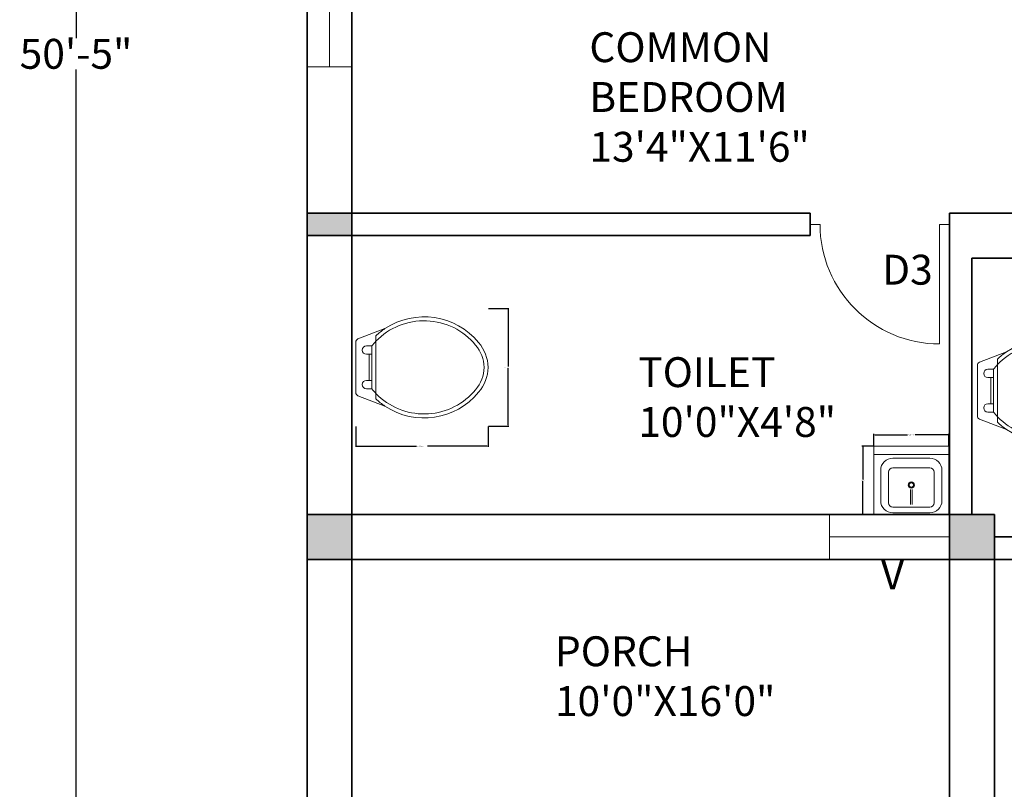
# Model space of a CAD drawing. Units: inches. Extents: x -36302355 to 648, y -221479757 to 75.
# Tile 12 of 37: x 87 to 285, y -425 to -271. Entities that reach past the tile are written whole.
import ezdxf

# ---------------------------------------------------------------- set-up
doc = ezdxf.new("R2010")
doc.units = ezdxf.units.IN
doc.header["$MEASUREMENT"] = 0
for name, color, linetype, lineweight in [('A-ANNO-DIMS', 2, 'Continuous', 18), ('A-ANNO-IDEN', 7, 'Continuous', 18), ('A-AREA-IDEN', 7, 'Continuous', 18), ('A-COLS', 7, 'Continuous', 35), ('A-COLS-PATT', 242, 'Continuous', 13), ('A-DOOR', 4, 'Continuous', 18), ('A-FLOR-FIXT', 9, 'Continuous', 18), ('A-GLAZ', 142, 'Continuous', 18), ('A-WALL', 7, 'Continuous', 35)]:
    doc.layers.add(name, color=color, linetype=linetype, lineweight=lineweight)
doc.styles.get("Standard").update_dxf_attribs({"font": 'arial.ttf'})
doc.dimstyles.get("Standard").update_dxf_attribs({"dimtxt": 0.18, "dimasz": 0.18, "dimexe": 0.18, "dimexo": 0.0625, "dimgap": 0.09, "dimtad": 0, "dimtih": 1, "dimtoh": 1, "dimdec": 0, "dimzin": 0, "dimdsep": 46, "dimlunit": 3, "dimtxsty": 'Standard', "dimcen": 0.09, "dimadec": 0, "dimazin": 0, "dimtfac": 1, "dimtdec": 0, "dimtofl": 0, "dimtmove": 0, "dimatfit": 3, "dimfxl": 1, "dimtolj": 1, "dimtzin": 0, "dimarcsym": 0})

# ---------------------------------------------------------------- blocks, each defined once
blk = doc.blocks.new('*D7')
at = {"layer": 'A-ANNO-DIMS', "color": 0, "lineweight": -2, "transparency": 16777216}
for p, q in [((145.13, 24.98), (98.63, 24.98)), ((98.81, 24.8), (98.81, -274.37)), ((98.81, -579.84), (98.81, -280.67)), ((145.13, -580.02), (98.63, -580.02))]:
    blk.add_line(p, q, dxfattribs=at)
at = {"layer": 'A-ANNO-DIMS', "color": 0, "transparency": 16777216}
for points in [[(98.78, 24.8), (98.84, 24.8), (98.81, 24.98)], [(98.78, -579.84), (98.84, -579.84), (98.81, -580.02)]]:
    blk.add_solid(points, dxfattribs=at)
at = {"layer": 'Defpoints', "color": 0, "transparency": 16777216}
for p in [(98.81, 24.98), (145.2, 24.98), (145.2, -580.02)]:
    blk.add_point(p, dxfattribs=at)
at = {"layer": 'A-ANNO-DIMS', "color": 0, "transparency": 16777216, "insert": (98.81, -277.52), "char_height": 6, "attachment_point": 5}
blk.add_mtext('\\A1;50\'-5"', dxfattribs=at)
blk = doc.blocks.new('М14 600х655')
for p, q in [((-655, 600), (-655, 0)), ((-655, 600), (-655, 0)), ((-655, 0), (-655, 600)), ((0, 600), (-655, 600)), ((0, 525), (-655, 525)), ((0, 0), (0, 600)), ((-165.1, 494.1), (-489.9, 494.1)), ((-595.8, 388.1), (-595.8, 121.3)), ((-528.4, 370.1), (-528.4, 103.3)), ((-165.4, 408.4), (-490.2, 408.4)), ((-127.2, 103.3), (-127.2, 370.1)), ((-59.2, 121.3), (-59.2, 388.1)), ((-333.5, 87.1), (-333.5, 219.6)), ((-321.5, 87.1), (-321.5, 219.6)), ((-655, 0), (-655, 0)), ((-655, 0), (-655, 0)), ((-655, 0), (0, 0)), ((-655, 0), (0, 0)), ((-490.2, 65.1), (-165.4, 65.1)), ((-489.9, 15.4), (-165.1, 15.4))]:
    blk.add_line(p, q)
for radius in [27.6, 19.3]:
    blk.add_circle((-327.5, 258.9), radius)
for centre, radius, start, end in [((-489.9, 388.1), 105.9, 90, 180), ((-165.1, 388.1), 105.9, 0, 90), ((-490.2, 370.1), 38.2, 90, 180), ((-165.4, 370.1), 38.2, 0, 90), ((-489.9, 121.3), 105.9, 180, 270), ((-490.2, 103.3), 38.2, 180, 270), ((-165.4, 103.3), 38.2, 270, 0), ((-165.1, 121.3), 105.9, 270, 0)]:
    blk.add_arc(centre, radius, start, end)
blk = doc.blocks.new('WC-FLOOR-MOUNT')
for p, q in [((4.02, 15.38), (4.02, 16.49)), ((4.02, 15.38), (4.02, 10.15)), ((4.02, 4.92), (4.02, 10.15)), ((4.02, 3.8), (4.02, 4.92))]:
    blk.add_line(p, q)
for points in [[(5.85, 17.93, -0.383919), (24.66, 15.14, -0.163732), (26.58, 10.15, -0.359733)], [(0, 10.15), (0, 15.22, -0.31031), (0.43, 15.85), (5.85, 17.93, -0.209071)], [(4.02, 15.38, -0.448546), (24.05, 14.64, -0.162618), (25.78, 10.15, -0.470877)], [(4.02, 16.49, -0.040937), (5.85, 17.93, -0.163732)], [(3.22, 14.46), (2.11, 14.46, 1), (2.11, 12.77), (2.69, 12.77)], [(3.22, 14.46, -0.022712), (4.02, 15.38, -0.162618)], [(3.22, 10.15), (3.22, 14.46, -0.476108)], [(0, 10.15), (0, 5.07, 0.31031), (0.43, 4.45), (5.85, 2.37, 0.209071)], [(3.22, 10.15), (3.22, 5.84, 0.022712)], [(4.57, 4.39, 0.431639), (24.05, 5.66, 0.162618), (25.78, 10.15, 0.470877)], [(5.85, 2.37, 0.383919), (24.66, 5.15, 0.163732), (26.58, 10.15, 0.359733)], [(3.22, 5.84), (2.11, 5.84, -1), (2.11, 7.53), (2.69, 7.53)], [(3.22, 5.84, 0.022712), (4.02, 4.92, 0.162618)], [(4.02, 4.92, 0.014165), (4.57, 4.39, 0.162618)], [(4.02, 3.8, 0.040937), (5.85, 2.37, 0.163732)]]:
    blk.add_lwpolyline(points, format="xyb")
for points in [[(2.69, 12.77), (2.69, 7.53)], [(2.69, 12.77), (3.22, 12.77)], [(2.69, 7.53), (3.22, 7.53)]]:
    blk.add_lwpolyline(points)
blk = doc.blocks.new('WIN-60')
for p, q in [((60, 9), (0, 9)), ((0, 9), (0, 0)), ((60, 0), (60, 9)), ((0, 4.5), (60, 4.5)), ((0, 0), (60, 0))]:
    blk.add_line(p, q)
blk = doc.blocks.new('VENT-24')
for p, q in [((0, 0), (0, 24)), ((0, 24), (9, 24)), ((4.5, 24), (4.5, 0)), ((9, 24), (9, 0)), ((9, 0), (0, 0))]:
    blk.add_line(p, q)
blk = doc.blocks.new('DOOR-SWING-24')
for p, q in [((0, 26), (0, 28)), ((0, 0), (0, 2)), ((0, 2), (24, 2))]:
    blk.add_line(p, q)
blk.add_arc((0, 2), 24, 0, 90)
blk = doc.blocks.new('*D31')
at = {"layer": 'A-ANNO-DIMS', "color": 0, "lineweight": -2, "transparency": 16777216}
for p, q in [((259.03, -356.21), (259.03, -353.84)), ((274.03, -356.21), (274.03, -353.84)), ((259.21, -354.02), (265.79, -354.02)), ((273.85, -354.02), (267.27, -354.02))]:
    blk.add_line(p, q, dxfattribs=at)
at = {"layer": 'A-ANNO-DIMS', "color": 0, "transparency": 16777216}
for points in [[(259.21, -353.99), (259.21, -354.05), (259.03, -354.02)], [(273.85, -353.99), (273.85, -354.05), (274.03, -354.02)]]:
    blk.add_solid(points, dxfattribs=at)
at = {"layer": 'Defpoints', "color": 0, "transparency": 16777216}
for p in [(274.03, -354.02), (259.03, -356.27), (274.03, -356.27)]:
    blk.add_point(p, dxfattribs=at)
at = {"layer": 'A-ANNO-DIMS', "color": 0, "transparency": 16777216, "insert": (266.53, -354.02), "char_height": 0.18, "attachment_point": 5}
blk.add_mtext('\\A1;BASIN 1\'-3"', dxfattribs=at)
blk = doc.blocks.new('*D32')
at = {"layer": 'A-ANNO-DIMS', "color": 0, "lineweight": -2, "transparency": 16777216}
for p, q in [((258.96, -356.27), (256.59, -356.27)), ((256.77, -356.45), (256.77, -362.96)), ((256.77, -369.84), (256.77, -363.33)), ((258.96, -370.02), (256.59, -370.02))]:
    blk.add_line(p, q, dxfattribs=at)
at = {"layer": 'A-ANNO-DIMS', "color": 0, "transparency": 16777216}
for points in [[(256.74, -356.45), (256.8, -356.45), (256.77, -356.27)], [(256.74, -369.84), (256.8, -369.84), (256.77, -370.02)]]:
    blk.add_solid(points, dxfattribs=at)
at = {"layer": 'Defpoints', "color": 0, "transparency": 16777216}
for p in [(256.77, -356.27), (259.03, -356.27), (259.03, -370.02)]:
    blk.add_point(p, dxfattribs=at)
at = {"layer": 'A-ANNO-DIMS', "color": 0, "transparency": 16777216, "insert": (256.77, -363.15), "char_height": 0.18, "attachment_point": 5}
blk.add_mtext('\\A1;1\'-1 1/2"', dxfattribs=at)
blk = doc.blocks.new('*D39')
at = {"layer": 'A-ANNO-DIMS', "color": 0, "lineweight": -2, "transparency": 16777216}
for p, q in [((154.99, -352.34), (154.99, -356.45)), ((181.57, -352.34), (181.57, -356.45)), ((155.17, -356.27), (167.19, -356.27)), ((181.39, -356.27), (169.38, -356.27))]:
    blk.add_line(p, q, dxfattribs=at)
at = {"layer": 'A-ANNO-DIMS', "color": 0, "transparency": 16777216}
for points in [[(155.17, -356.24), (155.17, -356.3), (154.99, -356.27)], [(181.39, -356.24), (181.39, -356.3), (181.57, -356.27)]]:
    blk.add_solid(points, dxfattribs=at)
at = {"layer": 'Defpoints', "color": 0, "transparency": 16777216}
for p in [(154.99, -352.28), (181.57, -352.28), (181.57, -356.27)]:
    blk.add_point(p, dxfattribs=at)
at = {"layer": 'A-ANNO-DIMS', "color": 0, "transparency": 16777216, "insert": (168.28, -356.27), "char_height": 0.18, "attachment_point": 5}
blk.add_mtext('\\A1;WC 2\'-2 1/2" TYP.', dxfattribs=at)
blk = doc.blocks.new('*D40')
at = {"layer": 'A-ANNO-DIMS', "color": 0, "lineweight": -2, "transparency": 16777216}
for p, q in [((181.64, -328.67), (185.74, -328.67)), ((185.56, -328.85), (185.56, -340.29)), ((185.56, -352.1), (185.56, -340.66)), ((181.64, -352.28), (185.74, -352.28))]:
    blk.add_line(p, q, dxfattribs=at)
at = {"layer": 'A-ANNO-DIMS', "color": 0, "transparency": 16777216}
for points in [[(185.53, -328.85), (185.59, -328.85), (185.56, -328.67)], [(185.53, -352.1), (185.59, -352.1), (185.56, -352.28)]]:
    blk.add_solid(points, dxfattribs=at)
at = {"layer": 'Defpoints', "color": 0, "transparency": 16777216}
for p in [(181.57, -328.67), (185.56, -328.67), (181.57, -352.28)]:
    blk.add_point(p, dxfattribs=at)
at = {"layer": 'A-ANNO-DIMS', "color": 0, "transparency": 16777216, "insert": (185.56, -340.47), "char_height": 0.18, "attachment_point": 5}
blk.add_mtext('\\A1;1\'-11 1/2" TYP.', dxfattribs=at)

msp = doc.modelspace()

# ---------------------------------------------------------------- hatches: boundary and pattern name
at = {"layer": 'A-COLS-PATT'}
h = msp.add_hatch(color=256, dxfattribs=at)
h.dxf.hatch_style = 1
h.paths.add_polyline_path([(145.2, 24.98), (145.2, 15.98), (154.2, 15.98), (154.2, 24.98)])
h.paths.add_polyline_path([(247.2, 15.98), (247.2, 24.98), (238.2, 24.98), (238.2, 15.98)])
h.paths.add_polyline_path([(387.64, 15.98), (395.7, 15.98), (395.7, 24.98), (387.64, 24.98)])
h.paths.add_polyline_path([(451.26, 24.98), (443.7, 24.98), (443.7, 15.98), (451.26, 15.98)])
h.paths.add_polyline_path([(596.2, 15.98), (605.2, 15.98), (605.2, 24.98), (596.2, 24.98)])
h.paths.add_polyline_path([(238.2, -122.02), (238.2, -131.02), (247.2, -131.02), (247.2, -122.02)])
h.paths.add_polyline_path([(395.7, -122.02), (387.46, -122.02), (387.46, -131.02), (395.7, -131.02)])
h.paths.add_polyline_path([(448.2, -131.02), (453.73, -131.02), (453.73, -122.02), (443.7, -122.02), (443.7, -131.02)])
h.paths.add_polyline_path([(596.2, -131.02), (605.2, -131.02), (605.2, -122.02), (596.2, -122.02)])
h.paths.add_polyline_path([(145.2, -176.97), (154.2, -176.97), (154.2, -167.02), (145.2, -167.02)])
h.paths.add_polyline_path([(314.2, -176.97), (323.2, -176.97), (323.2, -167.02), (314.2, -167.02)])
h.paths.add_polyline_path([(154.2, -314.02), (154.2, -309.52), (145.2, -309.52), (145.2, -314.02)])
h.paths.add_polyline_path([(314.2, -309.52), (314.2, -318.52), (323.2, -318.52), (323.2, -309.52)])
h.paths.add_polyline_path([(448.2, -277.02), (443.7, -277.02), (443.7, -286.02), (448.2, -286.02)])
h.paths.add_polyline_path([(283.2, -370.02), (274.2, -370.02), (274.2, -379.02), (283.2, -379.02), (283.2, -374.52)])
h.paths.add_polyline_path([(154.2, -370.02), (145.2, -370.02), (145.2, -379.02), (154.2, -379.02)])
h.paths.add_polyline_path([(443.2, -374.52), (443.2, -379.02), (452.2, -379.02), (452.2, -374.52)])
h.paths.add_polyline_path([(145.2, -580.02), (154.2, -580.02), (154.2, -571.02), (145.2, -571.02)])
h.paths.add_polyline_path([(274.2, -571.02), (274.2, -580.02), (283.2, -580.02), (283.2, -571.02)])
h.paths.add_polyline_path([(443.2, -580.02), (452.2, -580.02), (452.2, -571.02), (443.2, -571.02)])

# ---------------------------------------------------------------- linework, layer by layer
at = {"layer": 'A-COLS'}
for p, q in [((283.2, -370.02), (274.2, -370.02)), ((283.2, -374.52), (283.2, -370.02))]:
    msp.add_line(p, q, dxfattribs=at)
at = {"layer": 'A-WALL'}
for p, q in [((145.2, -167.02), (145.2, -722.02)), ((154.2, -167.02), (154.2, -722.02)), ((145.2, -309.52), (246.2, -309.52)), ((246.2, -311.77), (246.2, -309.52)), ((274.2, -309.52), (274.2, -580.02)), ((274.2, -309.52), (387.2, -309.52)), ((246.2, -311.77), (246.2, -314.02)), ((145.2, -314.02), (246.2, -314.02)), ((278.7, -318.52), (382.7, -318.52)), ((278.7, -318.52), (278.7, -370.02)), ((145.2, -370.02), (274.2, -370.02)), ((283.2, -374.52), (401.2, -374.52)), ((283.2, -374.52), (283.2, -580.02)), ((145.2, -379.02), (314.2, -379.02))]:
    msp.add_line(p, q, dxfattribs=at)

# ---------------------------------------------------------------- block references
at = {"layer": 'A-DOOR', "extrusion": (0, 0, -1), "zscale": -1, "rotation": 270}
msp.add_blockref('DOOR-SWING-24', (-274.2, -311.77), dxfattribs=at)
at = {"layer": 'A-FLOR-FIXT'}
for p in [(154.99, -350.62), (279.79, -355.3)]:
    msp.add_blockref('WC-FLOOR-MOUNT', p, dxfattribs=at)
at = {"layer": 'A-FLOR-FIXT', "xscale": 0.0229132871405827, "yscale": 0.0229132871405827, "zscale": 0.0229132871405827}
msp.add_blockref('М14 600х655', (274.03, -370.02), dxfattribs=at)
at = {"layer": 'A-GLAZ', "extrusion": (0, 0, -1), "zscale": -1, "rotation": 90}
for name, p in [('WIN-60', (-145.2, -280.1)), ('VENT-24', (-250.11, -379.02))]:
    msp.add_blockref(name, p, dxfattribs=at)

# ---------------------------------------------------------------- texts
at = {"layer": 'A-ANNO-IDEN', "char_height": 6, "attachment_point": 1}
for s, insert in [('D3', (260.65, -317.86)), ('V', (260.4, -379.02))]:
    msp.add_mtext(s, dxfattribs=dict(at, insert=insert))
at = {"layer": 'A-AREA-IDEN', "char_height": 6, "attachment_point": 1}
for s, insert in [('COMMON\\PBEDROOM\\P13\'4"X11\'6"', (201.88, -273.19)), ('PORCH\\P10\'0"X16\'0"', (194.97, -394.47))]:
    msp.add_mtext(s, dxfattribs=dict(at, insert=insert))
at = {"layer": 'A-AREA-IDEN', "insert": (211.7, -338.43), "char_height": 6, "attachment_point": 1}
msp.add_mtext_dynamic_manual_height_columns('TOILET\\P10\'0"X4\'8"', width=0.8076, gutter_width=1, heights=[0], dxfattribs=at)

# ---------------------------------------------------------------- dimensions: what is measured, and where the dimension line sits
at = {"layer": 'A-ANNO-DIMS'}
for base, p1, p2, override, picture, middle in [((98.81, 24.98), (145.2, -580.02), (145.2, 24.98), {"dimtxt": 6, "dimclrd": 0, "dimclre": 0, "dimclrt": 0}, '*D7', (98.81, -277.52)), ((256.7742, -356.2712), (259.0255, -370.0192), (259.0255, -356.2712), {"dimdec": 1, "dimlfac": 1, "dimrnd": 0, "dimzin": 1, "dimdsep": 46, "dimlunit": 4, "dimfrac": 2}, '*D32', (256.7742, -363.1452))]:
    dim = msp.add_linear_dim(base=base, p1=p1, p2=p2, angle=90, dimstyle='Standard', override=override, dxfattribs=at)
    dim.commit()
    dim.dimension.update_dxf_attribs({"geometry": picture, "text_midpoint": middle})
dim = msp.add_linear_dim(base=(185.56, -328.67), p1=(181.57, -352.28), p2=(181.57, -328.67), angle=90, text='<> TYP.', dimstyle='Standard', override={"dimdec": 1, "dimlfac": 1, "dimrnd": 0, "dimzin": 1, "dimdsep": 46, "dimlunit": 4, "dimfrac": 2}, dxfattribs=at)
dim.commit()
dim.dimension.update_dxf_attribs({"geometry": '*D40', "text_midpoint": (185.56, -340.47)})
for base, p1, p2, text, picture, middle in [((181.57, -356.27), (154.99, -352.28), (181.57, -352.28), 'WC <> TYP.', '*D39', (168.28, -356.27)), ((274.03, -354.02), (259.03, -356.27), (274.03, -356.27), 'BASIN <>', '*D31', (266.53, -354.02))]:
    dim = msp.add_linear_dim(base=base, p1=p1, p2=p2, text=text, dimstyle='Standard', override={"dimdec": 1, "dimlfac": 1, "dimrnd": 0, "dimzin": 1, "dimdsep": 46, "dimlunit": 4, "dimfrac": 2}, dxfattribs=at)
    dim.commit()
    dim.dimension.update_dxf_attribs({"geometry": picture, "text_midpoint": middle})

doc.saveas('drawing.dxf')
